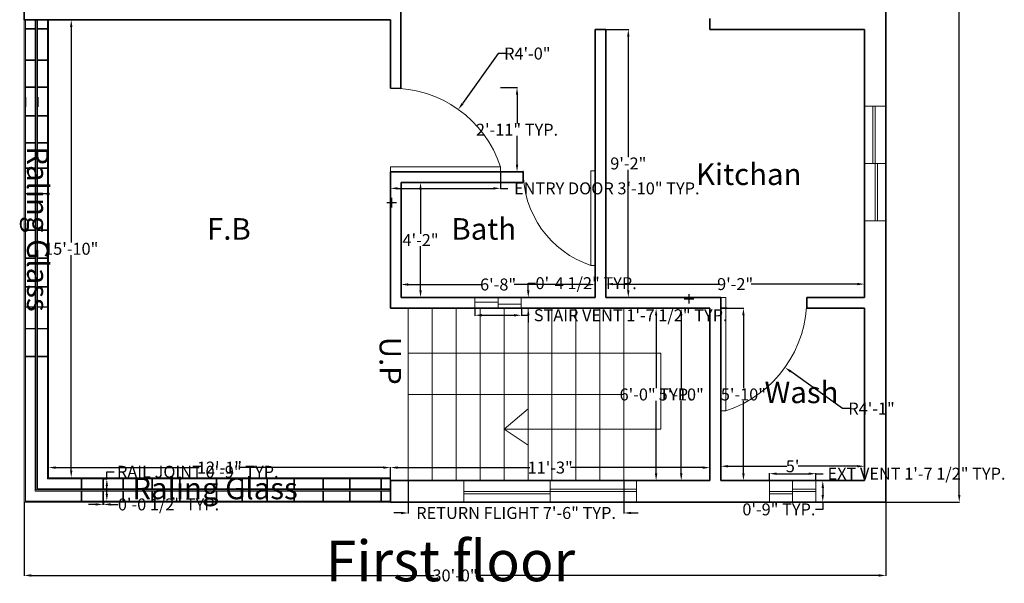
# Model space of a CAD drawing. Units: inches. Extents: x 534 to 1461, y 174 to 793.
# Tile 3 of 4: x 1050 to 1461, y 181 to 416. Entities that reach past the tile are written whole.
import ezdxf

# ---------------------------------------------------------------- set-up
doc = ezdxf.new("R2010")
doc.units = ezdxf.units.IN
doc.header["$MEASUREMENT"] = 0
for name, color, linetype, lineweight in [('A-ANNO-DIMS', 2, 'Continuous', 13), ('A-ANNO-SYMB', 7, 'Continuous', 15), ('A-FLOR-STRS', 7, 'Continuous', 18), ('A-GLAZ', 6, 'Continuous', 18), ('A-WALL', 7, 'Continuous', 35)]:
    doc.layers.add(name, color=color, linetype=linetype, lineweight=lineweight)
for name, color, linetype, lineweight, true_color in [('A-ANNO-TEXT', 254, 'Continuous', 18, 0xddb3d4), ('A-ANNO-TITL', 32, 'Continuous', 25, 0xcd6928), ('A-AREA-IDEN', 254, 'Continuous', 18, 0xddb3d4), ('A-DOOR', 165, 'Continuous', 20, 0x5e67af), ('A-FLOR-RAIL', 251, 'Continuous', 18, 0x636466)]:
    doc.layers.add(name, color=color, linetype=linetype, lineweight=lineweight, true_color=true_color)
doc.styles.get("Standard").update_dxf_attribs({"font": 'arial.ttf'})
doc.dimstyles.get("Standard").update_dxf_attribs({"dimtxt": 5, "dimasz": 3, "dimexe": 0.18, "dimexo": 0.0625, "dimgap": 0.09, "dimtad": 0, "dimtih": 1, "dimtoh": 1, "dimdec": 1, "dimrnd": 5, "dimzin": 0, "dimdsep": 46, "dimlunit": 4, "dimtxsty": 'Standard', "dimcen": 2, "dimclrd": 4, "dimclrt": 1, "dimadec": 0, "dimazin": 0, "dimtfac": 1, "dimtdec": 1, "dimtofl": 0, "dimtmove": 0, "dimatfit": 3, "dimfxl": 1, "dimtfillclr": 1, "dimtolj": 1, "dimtzin": 0, "dimarcsym": 0})

# ---------------------------------------------------------------- blocks, each defined once
blk = doc.blocks.new('*D41')
at = {"layer": 'A-ANNO-DIMS', "color": 0, "lineweight": -2, "transparency": 16777216}
for p, q in [((1209.53, 348), (1217.73, 348)), ((1217.55, 345), (1217.55, 326.6)), ((1217.55, 303), (1217.55, 321.4)), ((1209.53, 300), (1217.73, 300))]:
    blk.add_line(p, q, dxfattribs=at)
at = {"layer": 'A-ANNO-DIMS', "color": 0, "transparency": 16777216}
for points in [[(1217.05, 345), (1218.05, 345), (1217.55, 348)], [(1217.05, 303), (1218.05, 303), (1217.55, 300)]]:
    blk.add_solid(points, dxfattribs=at)
at = {"layer": 'Defpoints', "color": 0, "transparency": 16777216}
for p in [(1209.46, 348), (1209.46, 300), (1217.55, 300)]:
    blk.add_point(p, dxfattribs=at)
at = {"layer": 'A-ANNO-DIMS', "color": 0, "transparency": 16777216, "insert": (1217.55, 324), "char_height": 5, "attachment_point": 5}
blk.add_mtext('\\A1;4\'-2"', dxfattribs=at)
blk = doc.blocks.new('*D42')
at = {"layer": 'A-ANNO-DIMS', "color": 0, "lineweight": -2, "transparency": 16777216}
for p, q in [((1209.46, 300.06), (1209.46, 305.62)), ((1212.46, 305.44), (1243.21, 305.44)), ((1287.46, 305.44), (1256.71, 305.44)), ((1290.46, 300.06), (1290.46, 305.62))]:
    blk.add_line(p, q, dxfattribs=at)
at = {"layer": 'A-ANNO-DIMS', "color": 0, "transparency": 16777216}
for points in [[(1212.46, 305.94), (1212.46, 304.94), (1209.46, 305.44)], [(1287.46, 305.94), (1287.46, 304.94), (1290.46, 305.44)]]:
    blk.add_solid(points, dxfattribs=at)
at = {"layer": 'Defpoints', "color": 0, "transparency": 16777216}
for p in [(1290.46, 305.44), (1209.46, 300), (1290.46, 300)]:
    blk.add_point(p, dxfattribs=at)
at = {"layer": 'A-ANNO-DIMS', "color": 0, "transparency": 16777216, "insert": (1249.96, 305.44), "char_height": 5, "attachment_point": 5}
blk.add_mtext('\\A1;6\'-8"', dxfattribs=at)
blk = doc.blocks.new('*D43')
at = {"layer": 'A-ANNO-DIMS', "color": 0, "lineweight": -2, "transparency": 16777216}
for p, q in [((1295.03, 412), (1304.52, 412)), ((1304.34, 409), (1304.34, 358.64)), ((1304.34, 303), (1304.34, 353.36)), ((1295.03, 300), (1304.52, 300))]:
    blk.add_line(p, q, dxfattribs=at)
at = {"layer": 'A-ANNO-DIMS', "color": 0, "transparency": 16777216}
for points in [[(1303.84, 409), (1304.84, 409), (1304.34, 412)], [(1303.84, 303), (1304.84, 303), (1304.34, 300)]]:
    blk.add_solid(points, dxfattribs=at)
at = {"layer": 'Defpoints', "color": 0, "transparency": 16777216}
for p in [(1294.96, 412), (1294.96, 300), (1304.34, 300)]:
    blk.add_point(p, dxfattribs=at)
at = {"layer": 'A-ANNO-DIMS', "color": 0, "transparency": 16777216, "insert": (1304.34, 356), "char_height": 5, "attachment_point": 5}
blk.add_mtext('\\A1;9\'-2"', dxfattribs=at)
blk = doc.blocks.new('*D44')
at = {"layer": 'A-ANNO-DIMS', "color": 0, "lineweight": -2, "transparency": 16777216}
for p, q in [((1294.96, 300.06), (1294.96, 305.79)), ((1297.96, 305.61), (1342.23, 305.61)), ((1399.96, 305.61), (1355.7, 305.61)), ((1402.96, 300.06), (1402.96, 305.79))]:
    blk.add_line(p, q, dxfattribs=at)
at = {"layer": 'A-ANNO-DIMS', "color": 0, "transparency": 16777216}
for points in [[(1297.96, 306.11), (1297.96, 305.11), (1294.96, 305.61)], [(1399.96, 306.11), (1399.96, 305.11), (1402.96, 305.61)]]:
    blk.add_solid(points, dxfattribs=at)
at = {"layer": 'Defpoints', "color": 0, "transparency": 16777216}
for p in [(1402.96, 305.61), (1294.96, 300), (1402.96, 300)]:
    blk.add_point(p, dxfattribs=at)
at = {"layer": 'A-ANNO-DIMS', "color": 0, "transparency": 16777216, "insert": (1348.96, 305.61), "char_height": 5, "attachment_point": 5}
blk.add_mtext('\\A1;9\'-2"', dxfattribs=at)
blk = doc.blocks.new('*D45')
at = {"layer": 'A-ANNO-DIMS', "color": 0, "lineweight": -2, "transparency": 16777216}
for p, q in [((1343.03, 295.5), (1352.6, 295.5)), ((1352.42, 292.5), (1352.42, 262.14)), ((1352.42, 226.5), (1352.42, 256.86)), ((1343.03, 223.5), (1352.6, 223.5))]:
    blk.add_line(p, q, dxfattribs=at)
at = {"layer": 'A-ANNO-DIMS', "color": 0, "transparency": 16777216}
for points in [[(1351.92, 292.5), (1352.92, 292.5), (1352.42, 295.5)], [(1351.92, 226.5), (1352.92, 226.5), (1352.42, 223.5)]]:
    blk.add_solid(points, dxfattribs=at)
at = {"layer": 'Defpoints', "color": 0, "transparency": 16777216}
for p in [(1342.96, 295.5), (1342.96, 223.5), (1352.42, 223.5)]:
    blk.add_point(p, dxfattribs=at)
at = {"layer": 'A-ANNO-DIMS', "color": 0, "transparency": 16777216, "insert": (1352.42, 259.5), "char_height": 5, "attachment_point": 5}
blk.add_mtext('\\A1;5\'-10"', dxfattribs=at)
blk = doc.blocks.new('*D29')
at = {"layer": 'A-ANNO-DIMS', "color": 0, "lineweight": -2, "transparency": 16777216}
for p, q in [((1342.96, 223.56), (1342.96, 229.7)), ((1345.96, 229.52), (1370.57, 229.52)), ((1399.96, 229.52), (1375.35, 229.52)), ((1402.96, 223.56), (1402.96, 229.7))]:
    blk.add_line(p, q, dxfattribs=at)
at = {"layer": 'A-ANNO-DIMS', "color": 0, "transparency": 16777216}
for points in [[(1345.96, 230.02), (1345.96, 229.02), (1342.96, 229.52)], [(1399.96, 230.02), (1399.96, 229.02), (1402.96, 229.52)]]:
    blk.add_solid(points, dxfattribs=at)
at = {"layer": 'Defpoints', "color": 0, "transparency": 16777216}
for p in [(1402.96, 229.52), (1342.96, 223.5), (1402.96, 223.5)]:
    blk.add_point(p, dxfattribs=at)
at = {"layer": 'A-ANNO-DIMS', "color": 0, "transparency": 16777216, "insert": (1372.96, 229.52), "char_height": 5, "attachment_point": 5}
blk.add_mtext("\\A1;5'", dxfattribs=at)
blk = doc.blocks.new('*D30')
at = {"layer": 'A-ANNO-DIMS', "color": 0, "lineweight": -2, "transparency": 16777216}
for p, q in [((1338.4, 295.5), (1326.26, 295.5)), ((1326.44, 292.5), (1326.44, 262.14)), ((1326.44, 226.5), (1326.44, 256.86)), ((1338.4, 223.5), (1326.26, 223.5))]:
    blk.add_line(p, q, dxfattribs=at)
at = {"layer": 'A-ANNO-DIMS', "color": 0, "transparency": 16777216}
for points in [[(1325.94, 292.5), (1326.94, 292.5), (1326.44, 295.5)], [(1325.94, 226.5), (1326.94, 226.5), (1326.44, 223.5)]]:
    blk.add_solid(points, dxfattribs=at)
at = {"layer": 'Defpoints', "color": 0, "transparency": 16777216}
for p in [(1338.46, 295.5), (1326.44, 223.5), (1338.46, 223.5)]:
    blk.add_point(p, dxfattribs=at)
at = {"layer": 'A-ANNO-DIMS', "color": 0, "transparency": 16777216, "insert": (1326.44, 259.5), "char_height": 5, "attachment_point": 5}
blk.add_mtext('\\A1;5\'-10"', dxfattribs=at)
blk = doc.blocks.new('*D31')
at = {"layer": 'A-ANNO-DIMS', "color": 0, "lineweight": -2, "transparency": 16777216}
for p, q in [((1204.96, 223.56), (1204.96, 229.14)), ((1207.96, 228.96), (1263.27, 228.96)), ((1335.46, 228.96), (1280.16, 228.96)), ((1338.46, 223.56), (1338.46, 229.14))]:
    blk.add_line(p, q, dxfattribs=at)
at = {"layer": 'A-ANNO-DIMS', "color": 0, "transparency": 16777216}
for points in [[(1207.96, 229.46), (1207.96, 228.46), (1204.96, 228.96)], [(1335.46, 229.46), (1335.46, 228.46), (1338.46, 228.96)]]:
    blk.add_solid(points, dxfattribs=at)
at = {"layer": 'Defpoints', "color": 0, "transparency": 16777216}
for p in [(1338.46, 228.96), (1204.96, 223.5), (1338.46, 223.5)]:
    blk.add_point(p, dxfattribs=at)
at = {"layer": 'A-ANNO-DIMS', "color": 0, "transparency": 16777216, "insert": (1271.71, 228.96), "char_height": 5, "attachment_point": 5}
blk.add_mtext('\\A1;11\'-3"', dxfattribs=at)
blk = doc.blocks.new('*D49')
at = {"layer": 'A-ANNO-DIMS', "color": 0, "lineweight": -2, "transparency": 16777216}
for p, q in [((1062.26, 416), (1071.84, 416)), ((1071.66, 413), (1071.66, 323.01)), ((1071.66, 227.74), (1071.66, 317.73)), ((1062.26, 224.74), (1071.84, 224.74))]:
    blk.add_line(p, q, dxfattribs=at)
at = {"layer": 'A-ANNO-DIMS', "color": 0, "transparency": 16777216}
for points in [[(1071.16, 413), (1072.16, 413), (1071.66, 416)], [(1071.16, 227.74), (1072.16, 227.74), (1071.66, 224.74)]]:
    blk.add_solid(points, dxfattribs=at)
at = {"layer": 'Defpoints', "color": 0, "transparency": 16777216}
for p in [(1062.2, 416), (1062.2, 224.74), (1071.66, 224.74)]:
    blk.add_point(p, dxfattribs=at)
at = {"layer": 'A-ANNO-DIMS', "color": 0, "transparency": 16777216, "insert": (1071.66, 320.37), "char_height": 5, "attachment_point": 5}
blk.add_mtext('\\A1;15\'-10"', dxfattribs=at)
blk = doc.blocks.new('*D50')
at = {"layer": 'A-ANNO-DIMS', "color": 0, "lineweight": -2, "transparency": 16777216}
for p, q in [((1062.2, 224.8), (1062.2, 229.14)), ((1065.2, 228.96), (1125.14, 228.96)), ((1201.96, 228.96), (1142.03, 228.96)), ((1204.96, 224.8), (1204.96, 229.14))]:
    blk.add_line(p, q, dxfattribs=at)
at = {"layer": 'A-ANNO-DIMS', "color": 0, "transparency": 16777216}
for points in [[(1065.2, 229.46), (1065.2, 228.46), (1062.2, 228.96)], [(1201.96, 229.46), (1201.96, 228.46), (1204.96, 228.96)]]:
    blk.add_solid(points, dxfattribs=at)
at = {"layer": 'Defpoints', "color": 0, "transparency": 16777216}
for p in [(1204.96, 228.96), (1062.2, 224.74), (1204.96, 224.74)]:
    blk.add_point(p, dxfattribs=at)
at = {"layer": 'A-ANNO-DIMS', "color": 0, "transparency": 16777216, "insert": (1133.58, 228.96), "char_height": 5, "attachment_point": 5}
blk.add_mtext('\\A1;12\'-1"', dxfattribs=at)
blk = doc.blocks.new('WIN-SLIDING-48')
for p, q in [((0, 0), (0, 9)), ((24, 0), (24, 9)), ((48, 0), (48, 9)), ((0, 4.5), (48, 4.5)), ((24, 5.5), (48, 5.5)), ((0, 3.5), (24, 3.5))]:
    blk.add_line(p, q)
blk = doc.blocks.new('WIN-SLIDING-VENT-EXT')
for p, q in [((9, 19.38), (0, 19.38)), ((3.5, 19.38), (3.5, 9.69)), ((4.5, 19.38), (4.5, 0)), ((9, 9.69), (0, 9.69)), ((5.5, 9.69), (5.5, 0)), ((9, 0), (0, 0))]:
    blk.add_line(p, q)
blk = doc.blocks.new('WIN-SLIDING-VENT-STAIR')
for p, q in [((0, 0), (0, 4.5)), ((9.69, 0), (9.69, 4.5)), ((19.38, 0), (19.38, 4.5)), ((9.69, 2.58), (0, 2.58)), ((19.38, 0), (0, 0)), ((19.38, 1.76), (9.69, 1.76))]:
    blk.add_line(p, q)
blk = doc.blocks.new('WIN-SLIDING-72')
for p, q in [((0, 9), (0, 0)), ((36, 9), (36, 0)), ((72, 9), (72, 0)), ((0, 4.5), (72, 4.5)), ((36, 5.5), (72, 5.5)), ((0, 3.5), (36, 3.5))]:
    blk.add_line(p, q)
blk = doc.blocks.new('DOOR-SWING-BATH')
blk.add_lwpolyline([(30.07, 0), (28.27, 0), (28.27, 39.55), (30.07, 39.55)], close=True)
blk.add_arc((41.14, 39.08), 41.14, 179.344, 251.7744)
blk = doc.blocks.new('DOOR-SWING-ENTRY')
blk.add_lwpolyline([(45.99, 0), (45.99, 2.09), (0, 2.09), (0, 0)], close=True)
blk.add_arc((0.55, -12.87), 47.85, 18.2256, 90.656)
blk = doc.blocks.new('DOOR-SWING-WASH')
blk.add_lwpolyline([(0, 0), (2.15, 0), (2.15, 47.33), (0, 47.33)], close=True)
blk.add_arc((-13.25, 46.77), 49.24, 288.2256, 0.656)
blk = doc.blocks.new('STAIR-RETURN-FLIGHT')
for p, q in [((0, 72), (0, 0)), ((10, 72), (10, 0)), ((20, 72), (20, 0)), ((30, 72), (30, 0)), ((40, 72), (40, 0)), ((50, 72), (50, 0)), ((60, 72), (60, 0)), ((70, 72), (70, 0)), ((80, 72), (80, 0)), ((90, 72), (90, 0)), ((90, 36), (0, 36))]:
    blk.add_line(p, q)
blk = doc.blocks.new('ARROW-STAIR-RETURN')
for q in [(50, 15.21), (50, 0)]:
    blk.add_line((40, 6.74), q)
blk.add_lwpolyline([(0, 38.39), (105.42, 38.39), (105.42, 6.74), (40, 6.74)])
blk = doc.blocks.new('RAIL-GLASS-PANEL-JOINT')
for p, q in [((0, 9.24), (0, 5.12)), ((0.26, 9.24), (0.26, 5.12)), ((0, 4.12), (0, 0)), ((0.26, 4.12), (0.26, 0))]:
    blk.add_line(p, q)
blk = doc.blocks.new('*D73')
at = {"layer": 'A-ANNO-DIMS', "color": 0, "lineweight": -2, "transparency": 16777216}
for p, q in [((1363.27, 223.56), (1363.27, 226.59)), ((1382.66, 223.56), (1382.66, 226.59))]:
    blk.add_line(p, q, dxfattribs=at)
at = {"layer": 'A-ANNO-DIMS', "color": 4, "lineweight": -2, "transparency": 16777216}
for p, q in [((1366.27, 226.41), (1379.66, 226.41)), ((1382.66, 226.41), (1385.66, 226.41))]:
    blk.add_line(p, q, dxfattribs=at)
at = {"layer": 'A-ANNO-DIMS', "color": 4, "transparency": 16777216}
for points in [[(1366.27, 226.91), (1366.27, 225.91), (1363.27, 226.41)], [(1379.66, 226.91), (1379.66, 225.91), (1382.66, 226.41)]]:
    blk.add_solid(points, dxfattribs=at)
at = {"layer": 'Defpoints', "color": 0, "transparency": 16777216}
for p in [(1382.66, 226.41), (1363.27, 223.5), (1382.66, 223.5)]:
    blk.add_point(p, dxfattribs=at)
at = {"layer": 'A-ANNO-DIMS', "color": 1, "transparency": 16777216, "insert": (1424.73, 226.41), "char_height": 5, "attachment_point": 5}
blk.add_mtext('\\A1;EXT VENT 1\'-7 1/2" TYP.', dxfattribs=at)
blk = doc.blocks.new('*D74')
at = {"layer": 'A-ANNO-DIMS', "color": 0, "lineweight": -2, "transparency": 16777216}
for p, q in [((1382.72, 223.5), (1385.74, 223.5)), ((1382.72, 214.5), (1385.74, 214.5))]:
    blk.add_line(p, q, dxfattribs=at)
at = {"layer": 'A-ANNO-DIMS', "color": 4, "lineweight": -2, "transparency": 16777216}
for p, q in [((1385.56, 220.5), (1385.56, 217.5)), ((1385.56, 214.5), (1385.56, 211.5)), ((1385.56, 211.5), (1382.56, 211.5))]:
    blk.add_line(p, q, dxfattribs=at)
at = {"layer": 'A-ANNO-DIMS', "color": 4, "transparency": 16777216}
for points in [[(1385.06, 220.5), (1386.06, 220.5), (1385.56, 223.5)], [(1385.06, 217.5), (1386.06, 217.5), (1385.56, 214.5)]]:
    blk.add_solid(points, dxfattribs=at)
at = {"layer": 'Defpoints', "color": 0, "transparency": 16777216}
for p in [(1382.66, 223.5), (1382.66, 214.5), (1385.56, 214.5)]:
    blk.add_point(p, dxfattribs=at)
at = {"layer": 'A-ANNO-DIMS', "color": 1, "transparency": 16777216, "insert": (1367.24, 211.5), "char_height": 5, "attachment_point": 5}
blk.add_mtext('\\A1;0\'-9" TYP.', dxfattribs=at)
blk = doc.blocks.new('*D77')
at = {"layer": 'A-ANNO-DIMS', "color": 0, "lineweight": -2, "transparency": 16777216}
for p, q in [((1240.27, 295.44), (1240.27, 292.41)), ((1259.66, 295.44), (1259.66, 292.41))]:
    blk.add_line(p, q, dxfattribs=at)
at = {"layer": 'A-ANNO-DIMS', "color": 4, "lineweight": -2, "transparency": 16777216}
for p, q in [((1243.27, 292.59), (1256.66, 292.59)), ((1259.66, 292.59), (1262.66, 292.59))]:
    blk.add_line(p, q, dxfattribs=at)
at = {"layer": 'A-ANNO-DIMS', "color": 4, "transparency": 16777216}
for points in [[(1243.27, 293.09), (1243.27, 292.09), (1240.27, 292.59)], [(1256.66, 293.09), (1256.66, 292.09), (1259.66, 292.59)]]:
    blk.add_solid(points, dxfattribs=at)
at = {"layer": 'Defpoints', "color": 0, "transparency": 16777216}
for p in [(1240.27, 295.5), (1259.66, 295.5), (1259.66, 292.59)]:
    blk.add_point(p, dxfattribs=at)
at = {"layer": 'A-ANNO-DIMS', "color": 1, "transparency": 16777216, "insert": (1305.34, 292.59), "char_height": 5, "attachment_point": 5}
blk.add_mtext('\\A1;STAIR VENT 1\'-7 1/2" TYP.', dxfattribs=at)
blk = doc.blocks.new('*D78')
at = {"layer": 'A-ANNO-DIMS', "color": 4, "lineweight": -2, "transparency": 16777216}
for p, q in [((1262.56, 303), (1262.56, 306)), ((1262.56, 306), (1265.56, 306)), ((1262.56, 292.5), (1262.56, 289.5))]:
    blk.add_line(p, q, dxfattribs=at)
at = {"layer": 'A-ANNO-DIMS', "color": 0, "lineweight": -2, "transparency": 16777216}
for p, q in [((1259.72, 300), (1262.74, 300)), ((1259.72, 295.5), (1262.74, 295.5))]:
    blk.add_line(p, q, dxfattribs=at)
at = {"layer": 'A-ANNO-DIMS', "color": 4, "transparency": 16777216}
for points in [[(1262.06, 303), (1263.06, 303), (1262.56, 300)], [(1262.06, 292.5), (1263.06, 292.5), (1262.56, 295.5)]]:
    blk.add_solid(points, dxfattribs=at)
at = {"layer": 'Defpoints', "color": 0, "transparency": 16777216}
for p in [(1259.66, 300), (1262.56, 300), (1259.66, 295.5)]:
    blk.add_point(p, dxfattribs=at)
at = {"layer": 'A-ANNO-DIMS', "color": 1, "transparency": 16777216, "insert": (1286.72, 306), "char_height": 5, "attachment_point": 5}
blk.add_mtext('\\A1;0\'-4 1/2" TYP.', dxfattribs=at)
blk = doc.blocks.new('*D85')
at = {"layer": 'A-ANNO-DIMS', "color": 0, "lineweight": -2, "transparency": 16777216}
for p, q in [((1204.96, 352.44), (1204.96, 345.42)), ((1250.96, 352.44), (1250.96, 345.42))]:
    blk.add_line(p, q, dxfattribs=at)
at = {"layer": 'A-ANNO-DIMS', "color": 4, "lineweight": -2, "transparency": 16777216}
for p, q in [((1207.96, 345.6), (1247.96, 345.6)), ((1250.96, 345.6), (1253.96, 345.6))]:
    blk.add_line(p, q, dxfattribs=at)
at = {"layer": 'A-ANNO-DIMS', "color": 4, "transparency": 16777216}
for points in [[(1207.96, 346.1), (1207.96, 345.1), (1204.96, 345.6)], [(1247.96, 346.1), (1247.96, 345.1), (1250.96, 345.6)]]:
    blk.add_solid(points, dxfattribs=at)
at = {"layer": 'Defpoints', "color": 0, "transparency": 16777216}
for p in [(1204.96, 352.5), (1250.96, 352.5), (1250.96, 345.6)]:
    blk.add_point(p, dxfattribs=at)
at = {"layer": 'A-ANNO-DIMS', "color": 1, "transparency": 16777216, "insert": (1295.35, 345.6), "char_height": 5, "attachment_point": 5}
blk.add_mtext('\\A1;ENTRY DOOR 3\'-10" TYP.', dxfattribs=at)
blk = doc.blocks.new('*D86')
at = {"layer": 'A-ANNO-DIMS', "color": 0, "lineweight": -2, "transparency": 16777216}
for p, q in [((1251.02, 387.71), (1258.04, 387.71)), ((1251.02, 352.5), (1258.04, 352.5))]:
    blk.add_line(p, q, dxfattribs=at)
at = {"layer": 'A-ANNO-DIMS', "color": 4, "lineweight": -2, "transparency": 16777216}
for p, q in [((1257.86, 384.71), (1257.86, 372.71)), ((1257.86, 355.5), (1257.86, 367.5))]:
    blk.add_line(p, q, dxfattribs=at)
at = {"layer": 'A-ANNO-DIMS', "color": 4, "transparency": 16777216}
for points in [[(1257.36, 384.71), (1258.36, 384.71), (1257.86, 387.71)], [(1257.36, 355.5), (1258.36, 355.5), (1257.86, 352.5)]]:
    blk.add_solid(points, dxfattribs=at)
at = {"layer": 'Defpoints', "color": 0, "transparency": 16777216}
for p in [(1250.96, 387.71), (1257.86, 387.71), (1250.96, 352.5)]:
    blk.add_point(p, dxfattribs=at)
at = {"layer": 'A-ANNO-DIMS', "color": 1, "transparency": 16777216, "insert": (1257.86, 370.1), "char_height": 5, "attachment_point": 5}
blk.add_mtext('\\A1;2\'-11" TYP.', dxfattribs=at)
blk = doc.blocks.new('*D91')
at = {"layer": 'A-ANNO-DIMS', "color": 4, "lineweight": -2, "transparency": 16777216}
for p, q in [((1086.53, 224.2), (1086.53, 227.2)), ((1086.53, 227.2), (1089.53, 227.2)), ((1086.53, 217.97), (1086.53, 221.2))]:
    blk.add_line(p, q, dxfattribs=at)
at = {"layer": 'A-ANNO-DIMS', "color": 0, "lineweight": -2, "transparency": 16777216}
for p, q in [((1085.21, 224.2), (1086.71, 224.2)), ((1085.21, 214.97), (1086.71, 214.97))]:
    blk.add_line(p, q, dxfattribs=at)
at = {"layer": 'A-ANNO-DIMS', "color": 4, "transparency": 16777216}
for points in [[(1086.03, 221.2), (1087.03, 221.2), (1086.53, 224.2)], [(1086.03, 217.97), (1087.03, 217.97), (1086.53, 214.97)]]:
    blk.add_solid(points, dxfattribs=at)
at = {"layer": 'Defpoints', "color": 0, "transparency": 16777216}
for p in [(1085.15, 224.2), (1086.53, 224.2), (1085.15, 214.97)]:
    blk.add_point(p, dxfattribs=at)
at = {"layer": 'A-ANNO-DIMS', "color": 1, "transparency": 16777216, "insert": (1124.52, 227.2), "char_height": 5, "attachment_point": 5}
blk.add_mtext('\\A1;RAIL JOINT 0\'-9" TYP.', dxfattribs=at)
blk = doc.blocks.new('*D92')
at = {"layer": 'A-ANNO-DIMS', "color": 0, "lineweight": -2, "transparency": 16777216}
for p, q in [((1084.89, 214.9), (1084.89, 213.4)), ((1085.15, 214.9), (1085.15, 213.4))]:
    blk.add_line(p, q, dxfattribs=at)
at = {"layer": 'A-ANNO-DIMS', "color": 4, "lineweight": -2, "transparency": 16777216}
for p, q in [((1081.89, 213.58), (1078.89, 213.58)), ((1088.15, 213.58), (1091.15, 213.58))]:
    blk.add_line(p, q, dxfattribs=at)
at = {"layer": 'A-ANNO-DIMS', "color": 4, "transparency": 16777216}
for points in [[(1081.89, 214.08), (1081.89, 213.08), (1084.89, 213.58)], [(1088.15, 214.08), (1088.15, 213.08), (1085.15, 213.58)]]:
    blk.add_solid(points, dxfattribs=at)
at = {"layer": 'Defpoints', "color": 0, "transparency": 16777216}
for p in [(1084.89, 214.97), (1085.15, 214.97), (1085.15, 213.58)]:
    blk.add_point(p, dxfattribs=at)
at = {"layer": 'A-ANNO-DIMS', "color": 1, "transparency": 16777216, "insert": (1112.3, 213.58), "char_height": 5, "attachment_point": 5}
blk.add_mtext('\\A1;0\'-0 1/2" TYP.', dxfattribs=at)
blk = doc.blocks.new('*D93')
at = {"layer": 'A-ANNO-DIMS', "color": 0, "lineweight": -2, "transparency": 16777216}
for p, q in [((1212.46, 223.44), (1212.46, 209.82)), ((1302.46, 223.44), (1302.46, 209.82))]:
    blk.add_line(p, q, dxfattribs=at)
at = {"layer": 'A-ANNO-DIMS', "color": 4, "lineweight": -2, "transparency": 16777216}
for p, q in [((1209.46, 210), (1206.46, 210)), ((1305.46, 210), (1308.46, 210))]:
    blk.add_line(p, q, dxfattribs=at)
at = {"layer": 'A-ANNO-DIMS', "color": 4, "transparency": 16777216}
for points in [[(1209.46, 210.5), (1209.46, 209.5), (1212.46, 210)], [(1305.46, 210.5), (1305.46, 209.5), (1302.46, 210)]]:
    blk.add_solid(points, dxfattribs=at)
at = {"layer": 'Defpoints', "color": 0, "transparency": 16777216}
for p in [(1212.46, 223.5), (1302.46, 223.5), (1302.46, 210)]:
    blk.add_point(p, dxfattribs=at)
at = {"layer": 'A-ANNO-DIMS', "color": 1, "transparency": 16777216, "insert": (1257.46, 210), "char_height": 5, "attachment_point": 5}
blk.add_mtext('\\A1;RETURN FLIGHT 7\'-6" TYP.', dxfattribs=at)
blk = doc.blocks.new('*D94')
at = {"layer": 'A-ANNO-DIMS', "color": 0, "lineweight": -2, "transparency": 16777216}
for p, q in [((1302.53, 295.5), (1316.14, 295.5)), ((1302.53, 223.5), (1316.14, 223.5))]:
    blk.add_line(p, q, dxfattribs=at)
at = {"layer": 'A-ANNO-DIMS', "color": 4, "lineweight": -2, "transparency": 16777216}
for p, q in [((1315.96, 292.5), (1315.96, 262.14)), ((1315.96, 226.5), (1315.96, 256.86))]:
    blk.add_line(p, q, dxfattribs=at)
at = {"layer": 'A-ANNO-DIMS', "color": 4, "transparency": 16777216}
for points in [[(1315.46, 292.5), (1316.46, 292.5), (1315.96, 295.5)], [(1315.46, 226.5), (1316.46, 226.5), (1315.96, 223.5)]]:
    blk.add_solid(points, dxfattribs=at)
at = {"layer": 'Defpoints', "color": 0, "transparency": 16777216}
for p in [(1302.46, 295.5), (1315.96, 295.5), (1302.46, 223.5)]:
    blk.add_point(p, dxfattribs=at)
at = {"layer": 'A-ANNO-DIMS', "color": 1, "transparency": 16777216, "insert": (1315.96, 259.5), "char_height": 5, "attachment_point": 5}
blk.add_mtext('\\A1;6\'-0" TYP.', dxfattribs=at)
blk = doc.blocks.new('*D95')
at = {"layer": 'A-ANNO-DIMS', "color": 0, "lineweight": -2, "transparency": 16777216}
for p, q in [((1051.96, 214.44), (1051.96, 183.72)), ((1411.96, 214.44), (1411.96, 183.72))]:
    blk.add_line(p, q, dxfattribs=at)
at = {"layer": 'A-ANNO-DIMS', "color": 4, "lineweight": -2, "transparency": 16777216}
for p, q in [((1054.96, 183.9), (1223.29, 183.9)), ((1408.96, 183.9), (1240.64, 183.9))]:
    blk.add_line(p, q, dxfattribs=at)
at = {"layer": 'A-ANNO-DIMS', "color": 4, "transparency": 16777216}
for points in [[(1054.96, 184.4), (1054.96, 183.4), (1051.96, 183.9)], [(1408.96, 184.4), (1408.96, 183.4), (1411.96, 183.9)]]:
    blk.add_solid(points, dxfattribs=at)
at = {"layer": 'Defpoints', "color": 0, "transparency": 16777216}
for p in [(1051.96, 214.5), (1411.96, 214.5), (1411.96, 183.9)]:
    blk.add_point(p, dxfattribs=at)
at = {"layer": 'A-ANNO-DIMS', "color": 1, "transparency": 16777216, "insert": (1231.96, 183.9), "char_height": 5, "attachment_point": 5}
blk.add_mtext('\\A1;30\'-0"', dxfattribs=at)
blk = doc.blocks.new('*D96')
at = {"layer": 'A-ANNO-DIMS', "color": 0, "lineweight": -2, "transparency": 16777216}
for p, q in [((1412.03, 754.5), (1442.74, 754.5)), ((1412.03, 214.5), (1442.74, 214.5))]:
    blk.add_line(p, q, dxfattribs=at)
at = {"layer": 'A-ANNO-DIMS', "color": 4, "lineweight": -2, "transparency": 16777216}
for p, q in [((1442.56, 751.5), (1442.56, 487.14)), ((1442.56, 217.5), (1442.56, 481.86))]:
    blk.add_line(p, q, dxfattribs=at)
at = {"layer": 'A-ANNO-DIMS', "color": 4, "transparency": 16777216}
for points in [[(1442.06, 751.5), (1443.06, 751.5), (1442.56, 754.5)], [(1442.06, 217.5), (1443.06, 217.5), (1442.56, 214.5)]]:
    blk.add_solid(points, dxfattribs=at)
at = {"layer": 'Defpoints', "color": 0, "transparency": 16777216}
for p in [(1411.96, 754.5), (1442.56, 754.5), (1411.96, 214.5)]:
    blk.add_point(p, dxfattribs=at)
at = {"layer": 'A-ANNO-DIMS', "color": 1, "transparency": 16777216, "insert": (1442.56, 484.5), "char_height": 5, "attachment_point": 5}
blk.add_mtext('\\A1;45\'-0"', dxfattribs=at)
blk = doc.blocks.new('*D107')
at = {"layer": 'A-ANNO-DIMS', "color": 0, "lineweight": -2, "transparency": 16777216}
for p, q in [((1329.72, 297.44), (1329.72, 301.44)), ((1327.72, 299.44), (1331.72, 299.44))]:
    blk.add_line(p, q, dxfattribs=at)
at = {"layer": 'A-ANNO-DIMS', "color": 4, "lineweight": -2, "transparency": 16777216}
for p, q in [((1393.8, 253.62), (1372.21, 269.06)), ((1396.8, 253.62), (1393.8, 253.62))]:
    blk.add_line(p, q, dxfattribs=at)
at = {"layer": 'A-ANNO-DIMS', "color": 4, "transparency": 16777216}
blk.add_solid([(1372.5, 269.46), (1371.92, 268.65), (1369.77, 270.8)], dxfattribs=at)
at = {"layer": 'Defpoints', "color": 0, "transparency": 16777216}
for p in [(1329.72, 299.44), (1369.77, 270.8)]:
    blk.add_point(p, dxfattribs=at)
at = {"layer": 'A-ANNO-DIMS', "color": 1, "transparency": 16777216, "insert": (1405.93, 253.62), "char_height": 5, "attachment_point": 5}
blk.add_mtext('\\A1;R4\'-1"', dxfattribs=at)
blk = doc.blocks.new('*D113')
at = {"layer": 'A-ANNO-DIMS', "color": 4, "lineweight": -2, "transparency": 16777216}
for p, q in [((1250.03, 401.91), (1235.08, 380.99)), ((1253.03, 401.91), (1250.03, 401.91))]:
    blk.add_line(p, q, dxfattribs=at)
at = {"layer": 'A-ANNO-DIMS', "color": 0, "lineweight": -2, "transparency": 16777216}
for p, q in [((1205.51, 337.63), (1205.51, 341.63)), ((1203.51, 339.63), (1207.51, 339.63))]:
    blk.add_line(p, q, dxfattribs=at)
at = {"layer": 'A-ANNO-DIMS', "color": 4, "transparency": 16777216}
blk.add_solid([(1234.67, 381.28), (1235.49, 380.7), (1233.34, 378.55)], dxfattribs=at)
at = {"layer": 'Defpoints', "color": 0, "transparency": 16777216}
for p in [(1233.34, 378.55), (1205.51, 339.63)]:
    blk.add_point(p, dxfattribs=at)
at = {"layer": 'A-ANNO-DIMS', "color": 1, "transparency": 16777216, "insert": (1262.16, 401.91), "char_height": 5, "attachment_point": 5}
blk.add_mtext('\\A1;R4\'-0"', dxfattribs=at)

msp = doc.modelspace()

# ---------------------------------------------------------------- linework, layer by layer
at = {"layer": 'A-FLOR-RAIL'}
for p, q in [((1051.96, 416), (1051.96, 214.5)), ((1052.5, 416), (1052.5, 214.97)), ((1056.62, 416), (1056.62, 219.08)), ((1057.08, 416), (1057.08, 272)), ((1057.08, 416), (1057.08, 219.62)), ((1057.62, 416), (1057.62, 220.09)), ((1061.73, 416), (1061.73, 224.2)), ((1062.2, 416), (1062.2, 224.74)), ((1052.49, 383.76), (1052.49, 379.64)), ((1052.75, 383.76), (1052.75, 379.64)), ((1057.61, 383.76), (1057.61, 379.64)), ((1057.87, 383.76), (1057.87, 379.64)), ((1204.96, 219.62), (1204.96, 228.62)), ((1204.96, 224.2), (1061.73, 224.2)), ((1204.96, 224.74), (1062.2, 224.74)), ((1204.96, 219.08), (1056.62, 219.08)), ((1204.96, 219.62), (1057.08, 219.62)), ((1204.96, 220.09), (1057.62, 220.09)), ((1204.96, 219.62), (1060.96, 219.62)), ((1204.96, 214.5), (1051.96, 214.5)), ((1204.96, 214.97), (1052.5, 214.97))]:
    msp.add_line(p, q, dxfattribs=at)
at = {"layer": 'A-GLAZ'}
msp.add_line((1402.96, 356), (1411.96, 356), dxfattribs=at)
at = {"layer": 'A-WALL'}
for p, q in [((1051.96, 416), (1051.96, 754.5)), ((1411.96, 754.5), (1411.96, 214.5)), ((1209.37, 387.32), (1209.46, 549)), ((1051.96, 416), (1204.96, 416)), ((1204.97, 387.47), (1204.96, 416)), ((1338.46, 412), (1338.46, 416.5)), ((1290.46, 412), (1290.46, 300)), ((1290.46, 412), (1294.96, 412)), ((1294.96, 412), (1294.96, 300)), ((1402.96, 412), (1338.46, 412)), ((1402.96, 412), (1402.96, 300)), ((1209.37, 387.32), (1204.97, 387.47)), ((1260.46, 352.5), (1204.96, 352.5)), ((1204.96, 295.5), (1204.96, 352.5)), ((1260.46, 352.5), (1260.46, 348)), ((1260.46, 348), (1209.46, 348)), ((1209.46, 300), (1209.46, 348)), ((1290.46, 300), (1209.46, 300)), ((1342.96, 300), (1294.96, 300)), ((1342.96, 300), (1342.96, 223.5)), ((1378.96, 300), (1378.96, 295.5)), ((1402.96, 300), (1378.96, 300)), ((1338.46, 295.5), (1204.96, 295.5)), ((1338.46, 295.5), (1338.46, 223.5)), ((1345.57, 295.5), (1342.96, 295.5)), ((1402.96, 295.5), (1378.96, 295.5)), ((1402.96, 295.5), (1402.96, 223.5)), ((1338.46, 223.5), (1204.96, 223.5)), ((1204.96, 214.5), (1204.96, 223.5)), ((1402.96, 223.5), (1342.96, 223.5)), ((1411.96, 214.5), (1204.96, 214.5))]:
    msp.add_line(p, q, dxfattribs=at)

# ---------------------------------------------------------------- block references
at = {"layer": 'A-ANNO-SYMB'}
msp.add_blockref('ARROW-STAIR-RETURN', (1212.46, 238.32), dxfattribs=at)
at = {"layer": 'A-DOOR'}
for name, p in [('DOOR-SWING-ENTRY', (1204.96, 352.5)), ('DOOR-SWING-BATH', (1260.47, 313.42)), ('DOOR-SWING-WASH', (1342.96, 252.67))]:
    msp.add_blockref(name, p, dxfattribs=at)
at = {"layer": 'A-FLOR-RAIL'}
for p, rotation in [((1052.5, 412.32), 270.0000000000002), ((1052.5, 399.24), 270.0000000000002), ((1052.5, 388.05), 269.9999999999999), ((1052.5, 376), 269.9999999999995), ((1052.5, 364.71), 269.9999999999992), ((1052.5, 354.21), 269.9999999999999), ((1052.5, 343.51), 269.9999999999999), ((1052.5, 328.23), 269.9999999999993), ((1052.5, 316.61), 269.9999999999999), ((1052.5, 304.54), 270.0000000000002), ((1052.5, 296.18), 269.9999999999999), ((1052.5, 287.12), 269.9999999999993), ((1052.5, 275.45), 269.9999999999999)]:
    msp.add_blockref('RAIL-GLASS-PANEL-JOINT', p, dxfattribs=dict(at, rotation=rotation))
for p in [(1075.82, 214.97), (1084.89, 214.97), (1093.24, 214.97), (1105.32, 214.97), (1116.93, 214.97), (1132.22, 214.97), (1142.92, 214.97), (1153.41, 214.97), (1164.7, 214.97), (1176.76, 214.97), (1187.95, 214.97), (1201.03, 214.97)]:
    msp.add_blockref('RAIL-GLASS-PANEL-JOINT', p, dxfattribs=at)
at = {"layer": 'A-FLOR-STRS'}
msp.add_blockref('STAIR-RETURN-FLIGHT', (1212.46, 223.5), dxfattribs=at)
at = {"layer": 'A-GLAZ'}
for name, p, rotation in [('WIN-SLIDING-48', (1402.96, 380), 270.0000000000011), ('WIN-SLIDING-72', (1307.71, 223.5), 180), ('WIN-SLIDING-VENT-EXT', (1363.27, 223.5), 270.0000000000007)]:
    msp.add_blockref(name, p, dxfattribs=dict(at, rotation=rotation))
msp.add_blockref('WIN-SLIDING-VENT-STAIR', (1240.27, 295.5), dxfattribs=at)

# ---------------------------------------------------------------- texts
at = {"layer": 'A-ANNO-TEXT', "char_height": 9, "attachment_point": 1, "rotation": 270}
for s, width, insert in [('\\pxqc;Raling Glass ', 79.6518, (1062.2, 368.44)), ('\\pxqc;U.P', 52.8697, (1209.46, 300))]:
    msp.add_mtext_dynamic_manual_height_columns(s, width=width, gutter_width=1, heights=[0], dxfattribs=dict(at, insert=insert))
at = {"layer": 'A-ANNO-TEXT', "insert": (1091.91, 224.74), "char_height": 9, "attachment_point": 1}
msp.add_mtext_dynamic_manual_height_columns('\\pxqc;Raling Glass ', width=79.6518, gutter_width=1, heights=[0], dxfattribs=at)
at = {"layer": 'A-ANNO-TITL', "insert": (1168.1, 198.48), "char_height": 17, "attachment_point": 1}
msp.add_mtext_dynamic_manual_height_columns('\\pxqc;First floor ', width=123.8769, gutter_width=1, heights=[0], dxfattribs=at)
at = {"layer": 'A-AREA-IDEN', "char_height": 9, "attachment_point": 1}
for s, insert in [('\\pxqc;Kitchan ', (1328.2, 356)), ('\\pxqc;F.B', (1111.09, 333.15)), ('\\pxqc;Bath', (1217.55, 333.15)), ('\\pxqc;Wash ', (1350.24, 264.88))]:
    msp.add_mtext_dynamic_manual_height_columns(s, width=52.8697, gutter_width=1, heights=[0], dxfattribs=dict(at, insert=insert))

# ---------------------------------------------------------------- dimensions: what is measured, and where the dimension line sits
at = {"layer": 'A-ANNO-DIMS'}
for base, p1, p2, override, picture, middle in [((1442.56, 754.5), (1411.96, 214.5), (1411.96, 754.5), {"dimdec": 1, "dimlfac": 1, "dimrnd": 0, "dimzin": 1, "dimdsep": 46, "dimlunit": 4, "dimfrac": 2}, '*D96', (1442.56, 484.5)), ((1071.66, 224.74), (1062.2, 416), (1062.2, 224.74), {"dimclrd": 0, "dimclre": 0, "dimclrt": 0}, '*D49', (1071.66, 320.37)), ((1304.34, 300), (1294.96, 412), (1294.96, 300), {"dimclrd": 0, "dimclre": 0, "dimclrt": 0}, '*D43', (1304.34, 356)), ((1217.55, 300), (1209.46, 348), (1209.46, 300), {"dimclrd": 0, "dimclre": 0, "dimclrt": 0}, '*D41', (1217.55, 324)), ((1326.44, 223.5), (1338.46, 295.5), (1338.46, 223.5), {"dimclrd": 0, "dimclre": 0, "dimclrt": 0}, '*D30', (1326.44, 259.5)), ((1352.42, 223.5), (1342.96, 295.5), (1342.96, 223.5), {"dimclrd": 0, "dimclre": 0, "dimclrt": 0}, '*D45', (1352.42, 259.5))]:
    dim = msp.add_linear_dim(base=base, p1=p1, p2=p2, angle=90, dimstyle='Standard', override=override, dxfattribs=at)
    dim.commit()
    dim.dimension.update_dxf_attribs({"geometry": picture, "text_midpoint": middle})
for center, mpoint, picture, middle in [((1205.51, 339.63), (1233.34, 378.55), '*D113', (1262.16, 401.91)), ((1329.72, 299.44), (1369.77, 270.8), '*D107', (1405.93, 253.62))]:
    dim = msp.add_radius_dim(center=center, mpoint=mpoint, dimstyle='Standard', override={"dimdec": 1, "dimlfac": 1, "dimrnd": 0, "dimzin": 1, "dimdsep": 46, "dimlunit": 4, "dimfrac": 2}, dxfattribs=at)
    dim.commit()
    dim.dimension.update_dxf_attribs({"geometry": picture, "text_midpoint": middle, "dimtype": 164})
for base, p1, p2, angle, text, picture, middle in [((1257.86, 387.71), (1250.96, 352.5), (1250.96, 387.71), 90, '<> TYP.', '*D86', (1257.86, 370.1)), ((1262.56, 300), (1259.66, 295.5), (1259.66, 300), 90, '<> TYP.', '*D78', (1286.72, 306)), ((1315.96, 295.5), (1302.46, 223.5), (1302.46, 295.5), 90, '<> TYP.', '*D94', (1315.96, 259.5)), ((1086.53, 224.2), (1085.15, 214.97), (1085.15, 224.2), 90, 'RAIL JOINT <> TYP.', '*D91', (1124.52, 227.2)), ((1382.66, 226.41), (1363.27, 223.5), (1382.66, 223.5), 0, 'EXT VENT <> TYP.', '*D73', (1424.73, 226.41)), ((1385.56, 214.5), (1382.66, 223.5), (1382.66, 214.5), 270, '<> TYP.', '*D74', (1367.24, 211.5))]:
    dim = msp.add_linear_dim(base=base, p1=p1, p2=p2, angle=angle, text=text, dimstyle='Standard', override={"dimdec": 1, "dimlfac": 1, "dimrnd": 0, "dimzin": 1, "dimdsep": 46, "dimlunit": 4, "dimfrac": 2}, dxfattribs=at)
    dim.commit()
    dim.dimension.update_dxf_attribs({"geometry": picture, "text_midpoint": middle})
for base, p1, p2, text, picture, middle in [((1250.96, 345.6), (1204.96, 352.5), (1250.96, 352.5), 'ENTRY DOOR <> TYP.', '*D85', (1295.35, 345.6)), ((1259.66, 292.59), (1240.27, 295.5), (1259.66, 295.5), 'STAIR VENT <> TYP.', '*D77', (1305.34, 292.59)), ((1085.15, 213.58), (1084.89, 214.97), (1085.15, 214.97), '<> TYP.', '*D92', (1112.3, 213.58)), ((1302.46, 210), (1212.46, 223.5), (1302.46, 223.5), 'RETURN FLIGHT <> TYP.', '*D93', (1257.46, 210))]:
    dim = msp.add_linear_dim(base=base, p1=p1, p2=p2, text=text, dimstyle='Standard', override={"dimdec": 1, "dimlfac": 1, "dimrnd": 0, "dimzin": 1, "dimdsep": 46, "dimlunit": 4, "dimfrac": 2}, dxfattribs=at)
    dim.commit()
    dim.dimension.update_dxf_attribs({"geometry": picture, "text_midpoint": middle})
for base, p1, p2, override, picture, middle in [((1290.46, 305.44), (1209.46, 300), (1290.46, 300), {"dimclrd": 0, "dimclre": 0, "dimclrt": 0}, '*D42', (1249.96, 305.44)), ((1402.96, 305.61), (1294.96, 300), (1402.96, 300), {"dimclrd": 0, "dimclre": 0, "dimclrt": 0}, '*D44', (1348.96, 305.61)), ((1204.96, 228.96), (1062.2, 224.74), (1204.96, 224.74), {"dimclrd": 0, "dimclre": 0, "dimclrt": 0}, '*D50', (1133.58, 228.96)), ((1338.46, 228.96), (1204.96, 223.5), (1338.46, 223.5), {"dimclrd": 0, "dimclre": 0, "dimclrt": 0}, '*D31', (1271.71, 228.96)), ((1402.96, 229.52), (1342.96, 223.5), (1402.96, 223.5), {"dimclrd": 0, "dimclre": 0, "dimclrt": 0}, '*D29', (1372.96, 229.52)), ((1411.96, 183.9), (1051.96, 214.5), (1411.96, 214.5), {"dimdec": 1, "dimlfac": 1, "dimrnd": 0, "dimzin": 1, "dimdsep": 46, "dimlunit": 4, "dimfrac": 2}, '*D95', (1231.96, 183.9))]:
    dim = msp.add_linear_dim(base=base, p1=p1, p2=p2, dimstyle='Standard', override=override, dxfattribs=at)
    dim.commit()
    dim.dimension.update_dxf_attribs({"geometry": picture, "text_midpoint": middle})

doc.saveas('drawing.dxf')
